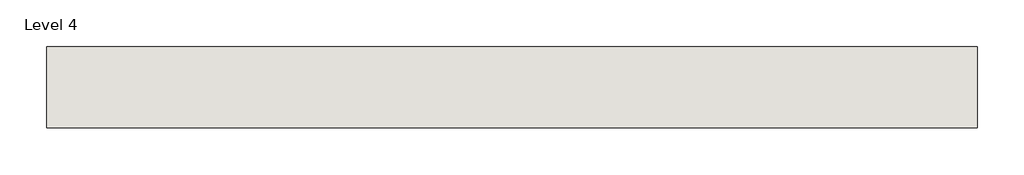
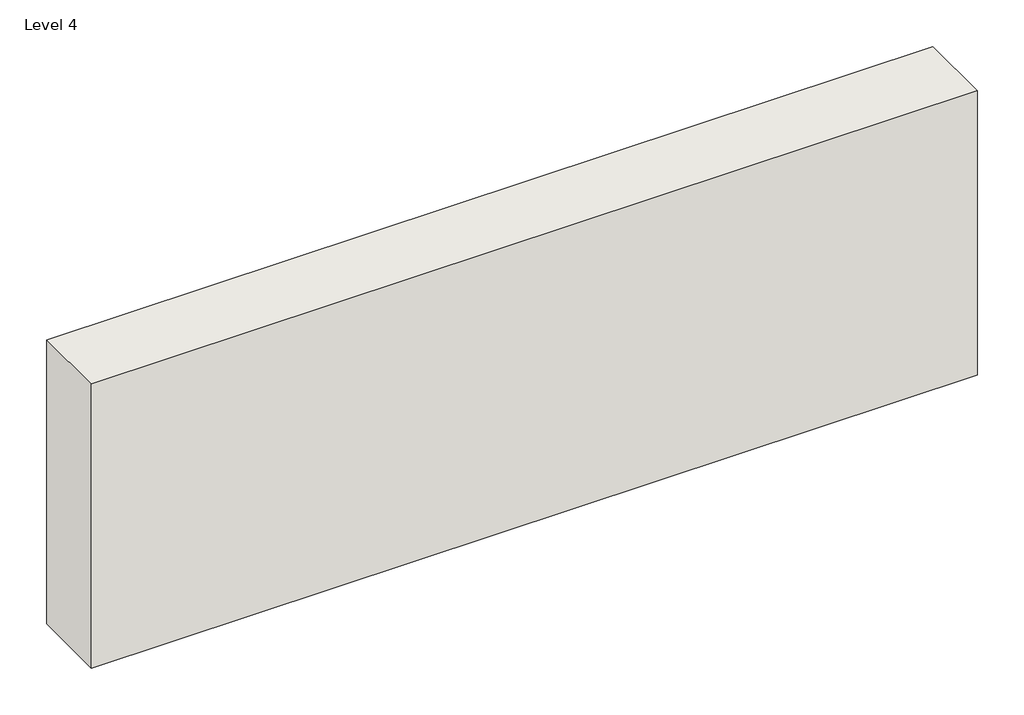
# One storey: 1 wall.
"""IFC4 building model written with IfcOpenShell, lengths in millimetres."""

from ifc_helpers import new_model, si_unit, frame, origin, place, context, project, spatial, polyline, outline, extrude, element, save

model = new_model("IFC4")

# Units and contexts
model_context = context("Model", 3, world=origin())
ifc_project = project(units=[si_unit("LENGTHUNIT", "METRE", prefix="MILLI")], contexts=[model_context])

# Site, building, storey
site = spatial("IfcSite", under=ifc_project)
building = spatial("IfcBuilding", under=site)
storey = spatial("IfcBuildingStorey", under=building, Name="Level 4", Elevation=10363.2)

# Wall
placement = place(None, origin())
element("IfcWall", 1, ObjectType="Generic - 12\"", at=placement, inside=storey, context=model_context, shape_type="SweptSolid", body=[
    extrude(outline(polyline([(-6964.1465329, 3890.6797737), (-10449.6306534, 3890.6797737), (-10449.6306534, 4195.4797737), (-6964.1465329, 4195.4797737), (-6964.1465329, 3890.6797737)])), frame((0.0, 0.0, 7213.6), z_axis=(0.0, 0.0, 1.0), x_axis=(1.0, 0.0, 0.0)), (0.0, 0.0, 1.0), 1182.8882518),
])

save(model, "model.ifc")

# Revit data of these elements
# Type "Generic - 12\""
#   Assembly Code = "B2010"
#   Layers, outside or top first: 1' - 0" no material (function 1)
# Element 1 (IfcWall, "Generic - 12\"")
#   built-in parameter 1001111 = -10' - 4"
#   Top Offset = 0' - 0"
#   Base Offset = -10' - 4"
#   Unconnected Height = 3' - 10.5704"
#   wall height = 3' - 10.5704"
#   Phase Created = New Construction
#   Base Constraint = Level 4
#   Materials on its faces: "Default Wall"
# Materials
#   "Default Wall": colour RGB 128 128 128, transparency 0
